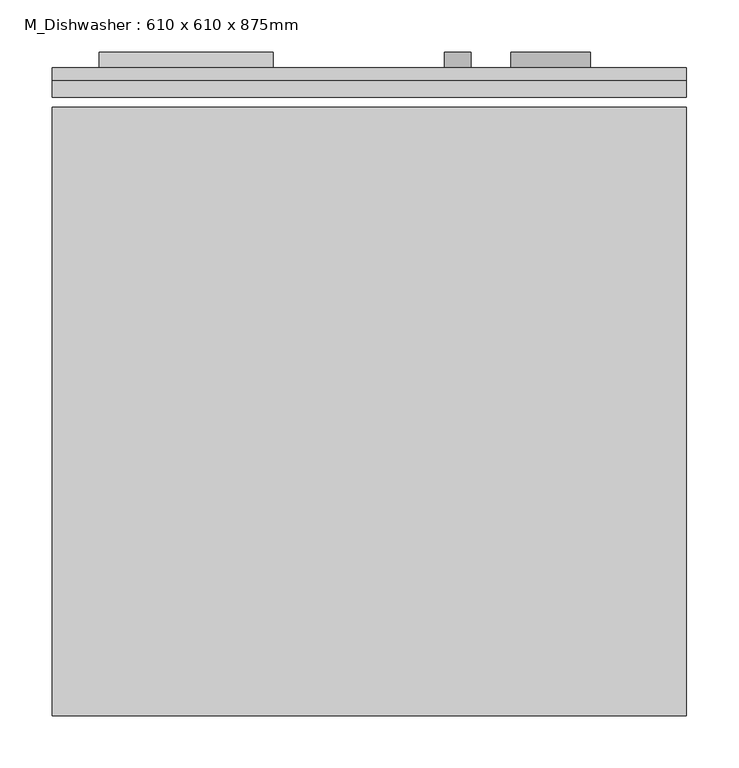
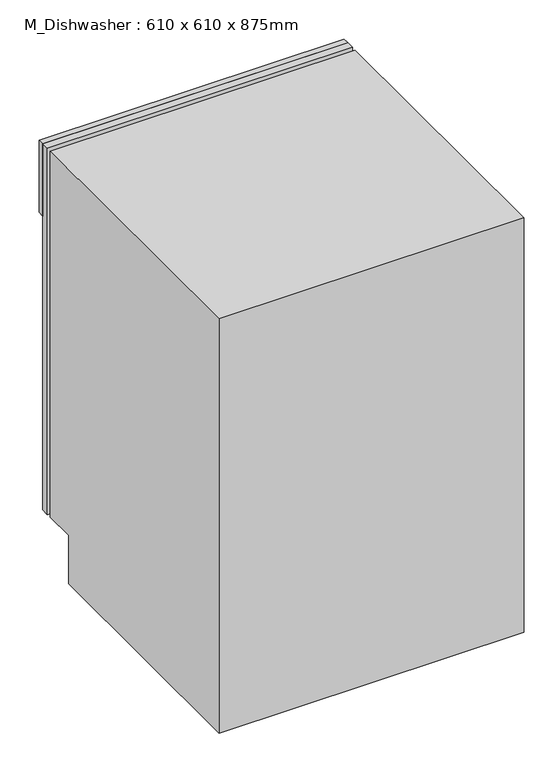
"""IFC4 building model written with IfcOpenShell, lengths in millimetres: proxy geometry, M_Dishwasher : 610 x 610 x 875mm."""

from ifc_helpers import new_model, si_unit, point, frame, frame_2d, origin, place, context, project, spatial, polyline, circle_curve, trimmed, segment, composite_curve, outline, extrude, source, transform, mapped, element, save


def m_dishwasher_610_x_610_x_875mm_75336c20(model_context):
    return source(origin(), model_context, "Body", "SweptSolid", [
        extrude(outline(polyline([(687.5174685, 38.3504352), (687.5174685, 22.4754352), (77.5174685, 22.4754352), (77.5174685, 38.3504352), (687.5174685, 38.3504352)])), frame((0.0, 0.0, 101.6), z_axis=(0.0, 0.0, 1.0), x_axis=(1.0, 0.0, 0.0)), (0.0, 0.0, 1.0), 773.4),
        extrude(outline(polyline([(687.5174685, 38.3504352), (77.5174685, 38.3504352), (77.5174685, 51.0504352), (687.5174685, 51.0504352), (687.5174685, 38.3504352)])), frame((0.0, 0.0, 722.6), z_axis=(0.0, 0.0, 1.0), x_axis=(1.0, 0.0, 0.0)), (0.0, 0.0, 1.0), 152.4),
        extrude(outline(polyline([(-571.6495648, 0.0), (-571.6495648, 875.0), (12.9504352, 875.0), (12.9504352, 101.6), (-50.5495648, 101.6), (-50.5495648, 0.0), (-571.6495648, 0.0)])), frame((77.5174685, 0.0, 0.0), z_axis=(1.0, 0.0, 0.0), x_axis=(0.0, 1.0, 0.0)), (0.0, 0.0, 1.0), 610.0),
        extrude(outline(polyline([(290.2347603, 66.0504352), (290.2347603, 51.0504352), (122.8347603, 51.0504352), (122.8347603, 66.0504352), (290.2347603, 66.0504352)])), frame((0.0, 0.0, 790.6663551), z_axis=(0.0, 0.0, 1.0), x_axis=(1.0, 0.0, 0.0)), (0.0, 0.0, 1.0), 50.8),
        extrude(outline(composite_curve([segment(trimmed(circle_curve(frame_2d((790.6663551, 467.3393328)), 12.7), [point((790.6663551, 480.0393328))], [point((790.6663551, 454.6393328))], False, "CARTESIAN"), True, "CONTINUOUS"), segment(trimmed(circle_curve(frame_2d((790.6663551, 467.3393328)), 12.7), [point((790.6663551, 454.6393328))], [point((790.6663551, 480.0393328))], False, "CARTESIAN"), True, "CONTINUOUS")], self_intersect=False)), frame((0.0, 51.0504352, 0.0), z_axis=(0.0, 1.0, 0.0), x_axis=(0.0, 0.0, 1.0)), (0.0, 0.0, 1.0), 15.0),
        extrude(outline(composite_curve([segment(trimmed(circle_curve(frame_2d((790.6663551, 556.7855874)), 38.1), [point((790.6663551, 594.8855874))], [point((790.6663551, 518.6855874))], False, "CARTESIAN"), True, "CONTINUOUS"), segment(trimmed(circle_curve(frame_2d((790.6663551, 556.7855874)), 38.1), [point((790.6663551, 518.6855874))], [point((790.6663551, 594.8855874))], False, "CARTESIAN"), True, "CONTINUOUS")], self_intersect=False)), frame((0.0, 51.0504352, 0.0), z_axis=(0.0, 1.0, 0.0), x_axis=(0.0, 0.0, 1.0)), (0.0, 0.0, 1.0), 15.0),
    ])


if __name__ == "__main__":
    model = new_model("IFC4")
    model_context = context("Model", 3, world=origin())
    ifc_project = project(units=[si_unit("LENGTHUNIT", "METRE", prefix="MILLI")], contexts=[model_context])
    site = spatial("IfcSite", under=ifc_project)
    building = spatial("IfcBuilding", under=site)
    placement = place(None, origin())
    m_dishwasher_610_x_610_x_875mm_shape = m_dishwasher_610_x_610_x_875mm_75336c20(model_context)
    element("IfcBuildingElementProxy", 1, Name="M_Dishwasher : 610 x 610 x 875mm", ObjectType="M_Dishwasher : 610 x 610 x 875mm", at=placement, inside=building, context=model_context, shape_type="MappedRepresentation", body=[
        mapped(m_dishwasher_610_x_610_x_875mm_shape, transform((0.0, 0.0, 0.0), x_axis=(1.0, 0.0, 0.0), y_axis=(0.0, 1.0, 0.0), z_axis=(0.0, 0.0, 1.0))),
    ])
    save(model, "model.ifc")

# Revit data of these elements
# Type "M_Dishwasher : 610 x 610 x 875mm"
#   Label = "DW"
#   Depth = 2.001312 ft
#   Height = 2.870735 ft
#   Width = 2.001312 ft
#   Dishwasher Material = Steel, Paint Finish, Ivory, Glossy
#   Panel Face Material = Plastic, Opaque Black
#   Default Elevation = 0
# Element 1 (IfcBuildingElementProxy, "M_Dishwasher : 610 x 610 x 875mm")
#   Materials on its faces: "Steel, Paint Finish, Ivory, Glossy", "Plastic, Opaque Black"
# Materials
#   "Steel, Paint Finish, Ivory, Glossy": class "Metal", colour RGB 247 247 239, transparency 0, Description = "Steel, paint finish, ivory, glossy", Cost = 0
#   "Plastic, Opaque Black": class "Plastic", colour RGB 0 0 0, transparency 0.7, Description = "Plastic, generic, opaque black", Cost = 0
